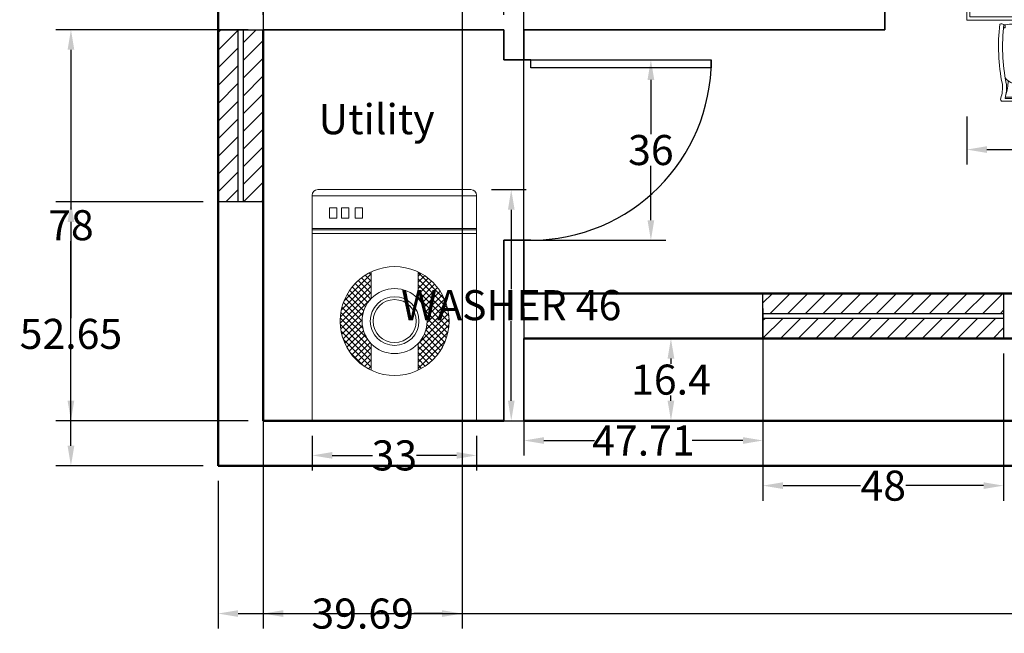
# Model space of a CAD drawing. Units: inches. Extents: x -1285 to -837, y -84 to 552.
# Tile 1 of 10: x -1285 to -1089, y -84 to 38. Entities that reach past the tile are written whole.
import ezdxf

# ---------------------------------------------------------------- set-up
doc = ezdxf.new("R2010")
doc.units = ezdxf.units.IN
doc.header["$MEASUREMENT"] = 0
for name, color, linetype, lineweight in [('A-ANNO-DIMS', 2, 'Continuous', 18), ('A-AREA-IDEN', 7, 'Continuous', 25), ('A-GLAZ-PATT', 191, 'Continuous', 13), ('Dining Table', 52, 'Continuous', 18), ('Doors', 34, 'Continuous', 25), ('Inner Wall', 202, 'Continuous', 35), ('Outer Wall', 12, 'Continuous', 50), ('Washing Machine', 133, 'Continuous', 18), ('Windows', 191, 'Continuous', 25)]:
    doc.layers.add(name, color=color, linetype=linetype, lineweight=lineweight)
doc.styles.get("Standard").update_dxf_attribs({"font": 'arial.ttf'})
doc.dimstyles.get("Standard").update_dxf_attribs({"dimtxt": 6, "dimasz": 4, "dimexe": 3, "dimexo": 3, "dimgap": 0.09, "dimtad": 0, "dimtih": 1, "dimtoh": 1, "dimdec": 1, "dimzin": 0, "dimdsep": 46, "dimlunit": 3, "dimtxsty": 'Standard', "dimcen": 0.09, "dimadec": 0, "dimazin": 0, "dimtfac": 1, "dimtdec": 1, "dimtofl": 0, "dimtmove": 0, "dimatfit": 3, "dimfxl": 1, "dimtolj": 1, "dimtzin": 0, "dimarcsym": 0})

# ---------------------------------------------------------------- blocks, each defined once
blk = doc.blocks.new('35')
for p, q in [((7268.4, 4404.4), (7268.4, 5204)), ((7288.4, 5224), (7831.6, 5224)), ((7851.6, 5204), (7851.6, 4404.4)), ((7268.4, 5201.6), (7851.6, 5201.6)), ((7329.8, 5159.5), (7355.7, 5159.5)), ((7329.8, 5122.5), (7329.8, 5159.5)), ((7355.7, 5159.5), (7355.7, 5122.5)), ((7372.4, 5159.5), (7398.4, 5159.5)), ((7372.4, 5122.5), (7372.4, 5159.5)), ((7398.4, 5159.5), (7398.4, 5122.5)), ((7420.7, 5159.5), (7446.7, 5159.5)), ((7420.7, 5122.5), (7420.7, 5159.5)), ((7446.7, 5159.5), (7446.7, 5122.5)), ((7355.7, 5122.5), (7329.8, 5122.5)), ((7398.4, 5122.5), (7372.4, 5122.5)), ((7446.7, 5122.5), (7420.7, 5122.5)), ((7268.4, 5085.6), (7851.6, 5085.6)), ((7268.4, 5080.8), (7851.6, 5080.8)), ((7268.4, 5068.6), (7851.6, 5068.6)), ((7381.6, 4829.3), (7477.8, 4925.5)), ((7477.8, 4921.2), (7470.7, 4928.4)), ((7477.8, 4837.6), (7477.8, 4932)), ((7644, 4837.6), (7644, 4932)), ((7737.2, 4836.4), (7644, 4929.6)), ((7644, 4917.1), (7653.8, 4926.9)), ((7372.1, 4798), (7477.8, 4903.7)), ((7418, 4887.6), (7431, 4900.5)), ((7476, 4835.7), (7421, 4890.8)), ((7477.8, 4855.8), (7432.1, 4901.5)), ((7477.8, 4877.6), (7444, 4911.4)), ((7477.8, 4899.4), (7456.9, 4920.3)), ((7644, 4895.3), (7667.4, 4918.7)), ((7644, 4873.5), (7680.1, 4909.6)), ((7748.5, 4803.3), (7644, 4907.8)), ((7644, 4851.7), (7691.9, 4899.5)), ((7368, 4750.2), (7477.8, 4860)), ((7368.4, 4772.5), (7477.8, 4881.9)), ((7458.1, 4810), (7401.5, 4866.6)), ((7466.3, 4823.6), (7410.8, 4879.1)), ((7753, 4777), (7644, 4886)), ((7753.9, 4754.2), (7644, 4864.2)), ((7647.7, 4833.6), (7702.8, 4888.6)), ((7657.2, 4821.2), (7712.8, 4876.8)), ((7665, 4807.2), (7722, 4864.2)), ((7369.8, 4730.2), (7477.8, 4838.2)), ((7445.6, 4757.1), (7379.3, 4823.3)), ((7447.2, 4777.2), (7385.7, 4838.8)), ((7451.7, 4794.6), (7393.1, 4853.2)), ((7752.5, 4733.8), (7644, 4842.3)), ((7671.1, 4791.5), (7730.2, 4850.6)), ((7675.1, 4773.7), (7737.4, 4836)), ((7676.1, 4752.8), (7743.5, 4820.3)), ((7464.3, 4694.7), (7370.3, 4788.7)), ((7373.3, 4711.9), (7449.7, 4788.3)), ((7448.4, 4732.4), (7374.1, 4806.7)), ((7644, 4677.1), (7752, 4785.1)), ((7749.3, 4715.3), (7670.3, 4794.2)), ((7672, 4727), (7748.5, 4803.4)), ((7477.8, 4659.4), (7368.2, 4769)), ((7378.3, 4695), (7445.7, 4762.5)), ((7644, 4655.3), (7753.8, 4765.1)), ((7744.6, 4698.1), (7675.9, 4766.8)), ((7477.8, 4637.6), (7368.1, 4747.3)), ((7477.8, 4615.7), (7371.1, 4722.5)), ((7384.4, 4679.4), (7446.7, 4741.7)), ((7391.6, 4664.8), (7450.7, 4723.8)), ((7644, 4633.4), (7753.4, 4742.9)), ((7644, 4611.6), (7749.7, 4717.3)), ((7731.6, 4667.4), (7672.1, 4727)), ((7738.6, 4682.2), (7675.6, 4745.3)), ((7477.8, 4593.9), (7379.1, 4692.6)), ((7399.9, 4651.2), (7456.8, 4708.1)), ((7409, 4638.5), (7464.7, 4694.1)), ((7419, 4626.7), (7474.1, 4681.8)), ((7644, 4589.8), (7740.2, 4686)), ((7704.7, 4628.9), (7649.6, 4684)), ((7714.6, 4640.8), (7658.7, 4696.7)), ((7723.6, 4653.7), (7666.3, 4710.9)), ((7450.9, 4599), (7402.3, 4647.6)), ((7430, 4615.8), (7477.8, 4663.6)), ((7477.8, 4583.4), (7477.8, 4677.7)), ((7644, 4583.4), (7644, 4677.7)), ((7694, 4617.8), (7644, 4667.8)), ((7682.3, 4607.6), (7644, 4645.9)), ((7441.7, 4605.8), (7477.8, 4641.8)), ((7454.4, 4596.6), (7477.8, 4620)), ((7669.8, 4598.3), (7644, 4624.1)), ((7691.5, 4615.5), (7703.1, 4627.1)), ((7468, 4588.4), (7477.8, 4598.2)), ((7656.4, 4589.9), (7644, 4602.3)), ((7851.6, 4404.4), (7268.4, 4404.4))]:
    blk.add_line(p, q)
for radius in [193.1, 115.3, 86.4, 76.4]:
    blk.add_circle((7560.9, 4757.7), radius)
for centre, start, end in [((7288.4, 5204), 90, 180), ((7831.6, 5204), 0, 90)]:
    blk.add_arc(centre, 20, start, end)
blk = doc.blocks.new('A$C51F1')
at = {"color": 0}
for p, q in [((0.2273, 0.4758), (0.0436, 0.4758)), ((0.2273, 0.4676), (0.0439, 0.4676)), ((0.2273, 0.4668), (0.0439, 0.4668)), ((0.2273, 0.4758), (0.4111, 0.4758)), ((0.2273, 0.4676), (0.4107, 0.4676)), ((0.2273, 0.4668), (0.4107, 0.4668)), ((0.2273, 0.3858), (0.1205, 0.3858)), ((0.2273, 0.3858), (0.3341, 0.3858)), ((0.0417, 0.0321), (0.0321, 0.0321)), ((0.0417, 0.0321), (0.0326, 0.0278)), ((0.0435, 0.0127), (0.0417, 0.0321)), ((0.4112, 0.0127), (0.4129, 0.0321)), ((0.4129, 0.0321), (0.4225, 0.0321)), ((0.4129, 0.0321), (0.4221, 0.0278))]:
    blk.add_line(p, q, dxfattribs=at)
blk.add_lwpolyline([(0.4387, 0.4737, 0.102523), (0.4291, 0.3863, -0.080461), (0.4447, 0.0091, -0.3023), (0.4203, 0.012, 0.197932), (0.4111, 0.0127, -0.028193), (0.3571, 0.0091), (0.227, 0.0091), (0.097, 0.0091, -0.028193), (0.0429, 0.0127, 0.197932), (0.0338, 0.012, -0.3023), (0.0093, 0.0091, -0.080461), (0.0249, 0.3863, 0.102523), (0.0153, 0.4737, -0.587111), (0.0261, 0.4929), (0.4279, 0.4929, -0.587111)], format="xyb", close=True, dxfattribs=at)
for centre, radius, start, end in [((0.044, 0.4735), 0.00242, 100.34496, 201.37417), ((-0.1898, 0.4063), 0.2409, 354.55133, 15.96258), ((0.0439, 0.4669), 0.000725, 87.37617, 197.52085), ((0.0438, 0.4664), 0.000433, 71.7715, 189.22024), ((-0.2563, 0.3584), 0.3173, 1.15909, 17.56409), ((0.7109, 0.3584), 0.3173, 162.43591, 178.84091), ((0.6445, 0.4063), 0.2409, 164.03742, 185.44867), ((0.4107, 0.4669), 0.000725, 342.47915, 92.62383), ((0.4109, 0.4664), 0.000433, 350.77976, 108.2285), ((0.4106, 0.4735), 0.00242, 338.62583, 79.65504), ((1.1806, 0.1494), 1.1544, 168.43567, 186.83625), ((0.1214, 0.2879), 0.0978, 90.51639, 143.19267), ((0.3332, 0.2879), 0.0978, 36.80733, 89.48361), ((-0.7259, 0.1494), 1.1544, 353.16375, 11.56433), ((0.0397, 0.0013), 0.012, 71.75361, 116.5375), ((0.4149, 0.0013), 0.012, 63.4625, 108.24639)]:
    blk.add_arc(centre, radius, start, end, dxfattribs=at)
blk = doc.blocks.new('Dining Table')
at = {"color": 0, "ltscale": 0.5}
for points in [[(5887.4, 1648.9), (7887.4, 1648.9), (7887.4, 2648.9), (5887.4, 2648.9)], [(5907.4, 1668.9), (7867.4, 1668.9), (7867.4, 2628.9), (5907.4, 2628.9)]]:
    blk.add_lwpolyline(points, close=True, dxfattribs=at)
at = {"color": 0, "ltscale": 0.5, "yscale": 1000, "zscale": 1000}
for p, xscale in [((6085.4, 2664.8), 1000), ((6685.4, 2664.8), 1000), ((7739.4, 2664.8), -1000)]:
    blk.add_blockref('A$C51F1', p, dxfattribs=dict(at, xscale=xscale))
at = {"color": 0, "ltscale": 0.5, "yscale": 1000, "zscale": 1000, "rotation": 180}
for p, xscale in [((6085.4, 1633), -1000), ((6685.4, 1633), -1000), ((7739.4, 1633), 1000)]:
    blk.add_blockref('A$C51F1', p, dxfattribs=dict(at, xscale=xscale))
blk = doc.blocks.new('*U17')
for p, q in [((-40, 0), (-40, 6)), ((0, 0), (0, 6))]:
    blk.add_line(p, q)
blk.add_lwpolyline([(0, 0), (0, -40), (-1.75, -40), (-1.75, 0)], close=True)
blk.add_arc((0, 0), 40, 180, 270)
blk = doc.blocks.new('WIN-34x9')
for p, q in [((4, 0), (4, 34.35)), ((5, 34.35), (5, 0))]:
    blk.add_line(p, q)
blk.add_lwpolyline([(9, 34.35), (9, 0), (0, 0), (0, 34.35)], close=True)
blk = doc.blocks.new('*D53')
at = {"layer": 'A-ANNO-DIMS', "color": 0, "lineweight": -2, "transparency": 16777216}
for p, q in [((-1190.95, 4.04), (-1184.04, 4.04)), ((-1187.04, 0.04), (-1187.04, -15.82)), ((-1187.04, -38.06), (-1187.04, -22.2)), ((-1190.95, -42.06), (-1184.04, -42.06))]:
    blk.add_line(p, q, dxfattribs=at)
at = {"layer": 'A-ANNO-DIMS', "color": 0, "transparency": 16777216}
for points in [[(-1187.7, 0.04), (-1186.37, 0.04), (-1187.04, 4.04)], [(-1187.7, -38.06), (-1186.37, -38.06), (-1187.04, -42.06)]]:
    blk.add_solid(points, dxfattribs=at)
at = {"layer": 'Defpoints', "color": 0, "transparency": 16777216}
for p in [(-1193.95, 4.04), (-1187.04, 4.04), (-1193.95, -42.06)]:
    blk.add_point(p, dxfattribs=at)
at = {"layer": 'A-ANNO-DIMS', "color": 0, "transparency": 16777216, "insert": (-1187.04, -19.01), "char_height": 6, "attachment_point": 5}
blk.add_mtext('\\A1;WASHER 46', dxfattribs=at)
blk = doc.blocks.new('*D54')
at = {"layer": 'A-ANNO-DIMS', "color": 0, "lineweight": -2, "transparency": 16777216}
for p, q in [((-1226.76, -45.06), (-1226.76, -51.98)), ((-1193.95, -45.06), (-1193.95, -51.98)), ((-1222.76, -48.98), (-1214.74, -48.98)), ((-1197.95, -48.98), (-1205.97, -48.98))]:
    blk.add_line(p, q, dxfattribs=at)
at = {"layer": 'A-ANNO-DIMS', "color": 0, "transparency": 16777216}
for points in [[(-1222.76, -48.31), (-1222.76, -49.64), (-1226.76, -48.98)], [(-1197.95, -48.31), (-1197.95, -49.64), (-1193.95, -48.98)]]:
    blk.add_solid(points, dxfattribs=at)
at = {"layer": 'Defpoints', "color": 0, "transparency": 16777216}
for p in [(-1226.76, -42.06), (-1193.95, -42.06), (-1193.95, -48.98)]:
    blk.add_point(p, dxfattribs=at)
at = {"layer": 'A-ANNO-DIMS', "color": 0, "transparency": 16777216, "insert": (-1210.36, -48.98), "char_height": 6, "attachment_point": 5}
blk.add_mtext('\\A1;33', dxfattribs=at)
blk = doc.blocks.new('*D58')
at = {"layer": 'A-ANNO-DIMS', "color": 0, "lineweight": -2, "transparency": 16777216}
for p, q in [((-1096.15, 18.66), (-1096.15, 9.03)), ((-1032.53, 18.66), (-1032.53, 9.03)), ((-1092.15, 12.03), (-1068.73, 12.03)), ((-1036.53, 12.03), (-1059.95, 12.03))]:
    blk.add_line(p, q, dxfattribs=at)
at = {"layer": 'A-ANNO-DIMS', "color": 0, "transparency": 16777216}
for points in [[(-1092.15, 12.7), (-1092.15, 11.36), (-1096.15, 12.03)], [(-1036.53, 12.7), (-1036.53, 11.36), (-1032.53, 12.03)]]:
    blk.add_solid(points, dxfattribs=at)
at = {"layer": 'Defpoints', "color": 0, "transparency": 16777216}
for p in [(-1096.15, 21.66), (-1032.53, 21.66), (-1032.53, 12.03)]:
    blk.add_point(p, dxfattribs=at)
at = {"layer": 'A-ANNO-DIMS', "color": 0, "transparency": 16777216, "insert": (-1064.34, 12.03), "char_height": 6, "attachment_point": 5}
blk.add_mtext('\\A1;64', dxfattribs=at)
blk = doc.blocks.new('*D69')
at = {"layer": 'A-ANNO-DIMS', "color": 0, "lineweight": -2, "transparency": 16777216}
for p, q in [((-1245.53, -54.06), (-1245.53, -83.53)), ((-877.53, -54.06), (-877.53, -83.53)), ((-1241.53, -80.53), (-1068.25, -80.53)), ((-881.53, -80.53), (-1054.81, -80.53))]:
    blk.add_line(p, q, dxfattribs=at)
at = {"layer": 'A-ANNO-DIMS', "color": 0, "transparency": 16777216}
for points in [[(-1241.53, -79.86), (-1241.53, -81.2), (-1245.53, -80.53)], [(-881.53, -79.86), (-881.53, -81.2), (-877.53, -80.53)]]:
    blk.add_solid(points, dxfattribs=at)
at = {"layer": 'Defpoints', "color": 0, "transparency": 16777216}
for p in [(-1245.53, -51.06), (-877.53, -51.06), (-877.53, -80.53)]:
    blk.add_point(p, dxfattribs=at)
at = {"layer": 'A-ANNO-DIMS', "color": 0, "transparency": 16777216, "insert": (-1061.53, -80.53), "char_height": 6, "attachment_point": 5}
blk.add_mtext('\\A1;368', dxfattribs=at)
blk = doc.blocks.new('*D77')
at = {"layer": 'A-ANNO-DIMS', "color": 0, "lineweight": -2, "transparency": 16777216}
for p, q in [((-1239.53, 35.94), (-1277.88, 35.94)), ((-1274.88, 31.94), (-1274.88, 0.09)), ((-1274.88, -38.06), (-1274.88, -6.21)), ((-1239.53, -42.06), (-1277.88, -42.06))]:
    blk.add_line(p, q, dxfattribs=at)
at = {"layer": 'A-ANNO-DIMS', "color": 0, "transparency": 16777216}
for points in [[(-1275.55, 31.94), (-1274.21, 31.94), (-1274.88, 35.94)], [(-1275.55, -38.06), (-1274.21, -38.06), (-1274.88, -42.06)]]:
    blk.add_solid(points, dxfattribs=at)
at = {"layer": 'Defpoints', "color": 0, "transparency": 16777216}
for p in [(-1274.88, 35.94), (-1236.53, 35.94), (-1236.53, -42.06)]:
    blk.add_point(p, dxfattribs=at)
at = {"layer": 'A-ANNO-DIMS', "color": 0, "transparency": 16777216, "insert": (-1274.88, -3.06), "char_height": 6, "attachment_point": 5}
blk.add_mtext('\\A1;78', dxfattribs=at)
blk = doc.blocks.new('*D79')
at = {"layer": 'A-ANNO-DIMS', "color": 0, "lineweight": -2, "transparency": 16777216}
for p, q in [((-1236.53, 38.94), (-1236.53, 551.29)), ((-1188.53, 38.94), (-1188.53, 551.29)), ((-1232.53, 548.29), (-1217.04, 548.29)), ((-1192.53, 548.29), (-1208.02, 548.29))]:
    blk.add_line(p, q, dxfattribs=at)
at = {"layer": 'A-ANNO-DIMS', "color": 0, "transparency": 16777216}
for points in [[(-1232.53, 548.96), (-1232.53, 547.62), (-1236.53, 548.29)], [(-1192.53, 548.96), (-1192.53, 547.62), (-1188.53, 548.29)]]:
    blk.add_solid(points, dxfattribs=at)
at = {"layer": 'Defpoints', "color": 0, "transparency": 16777216}
for p in [(-1188.53, 548.29), (-1236.53, 35.94), (-1188.53, 35.94)]:
    blk.add_point(p, dxfattribs=at)
at = {"layer": 'A-ANNO-DIMS', "color": 0, "transparency": 16777216, "insert": (-1212.53, 548.29), "char_height": 6, "attachment_point": 5}
blk.add_mtext('\\A1;48', dxfattribs=at)
blk = doc.blocks.new('*D80')
at = {"layer": 'A-ANNO-DIMS', "color": 0, "lineweight": -2, "transparency": 16777216}
for p, q in [((-1184.53, -13.66), (-1184.53, 551.29)), ((-1032.53, -13.66), (-1032.53, 551.29)), ((-1180.53, 548.29), (-1114.94, 548.29)), ((-1036.53, 548.29), (-1102.12, 548.29))]:
    blk.add_line(p, q, dxfattribs=at)
at = {"layer": 'A-ANNO-DIMS', "color": 0, "transparency": 16777216}
for points in [[(-1180.53, 548.96), (-1180.53, 547.62), (-1184.53, 548.29)], [(-1036.53, 548.96), (-1036.53, 547.62), (-1032.53, 548.29)]]:
    blk.add_solid(points, dxfattribs=at)
at = {"layer": 'Defpoints', "color": 0, "transparency": 16777216}
for p in [(-1032.53, 548.29), (-1184.53, -16.66), (-1032.53, -16.66)]:
    blk.add_point(p, dxfattribs=at)
at = {"layer": 'A-ANNO-DIMS', "color": 0, "transparency": 16777216, "insert": (-1108.53, 548.29), "char_height": 6, "attachment_point": 5}
blk.add_mtext('\\A1;152', dxfattribs=at)
blk = doc.blocks.new('*D96')
at = {"layer": 'A-ANNO-DIMS', "color": 0, "lineweight": -2, "transparency": 16777216}
for p, q in [((-1236.53, 506.94), (-1236.53, -83.53)), ((-1196.84, 506.94), (-1196.84, -83.53)), ((-1232.53, -80.53), (-1226.9, -80.53)), ((-1200.84, -80.53), (-1206.47, -80.53))]:
    blk.add_line(p, q, dxfattribs=at)
at = {"layer": 'A-ANNO-DIMS', "color": 0, "transparency": 16777216}
for points in [[(-1232.53, -79.86), (-1232.53, -81.2), (-1236.53, -80.53)], [(-1200.84, -79.86), (-1200.84, -81.2), (-1196.84, -80.53)]]:
    blk.add_solid(points, dxfattribs=at)
at = {"layer": 'Defpoints', "color": 0, "transparency": 16777216}
for p in [(-1236.53, 509.94), (-1196.84, 509.94), (-1196.84, -80.53)]:
    blk.add_point(p, dxfattribs=at)
at = {"layer": 'A-ANNO-DIMS', "color": 0, "transparency": 16777216, "insert": (-1216.68, -80.53), "char_height": 6, "attachment_point": 5}
blk.add_mtext('\\A1;39.69', dxfattribs=at)
blk = doc.blocks.new('*D100')
at = {"layer": 'A-ANNO-DIMS', "color": 0, "lineweight": -2, "transparency": 16777216}
for p, q in [((-1184.53, -19.66), (-1184.53, -49.01)), ((-1136.82, -19.66), (-1136.82, -49.01)), ((-1180.53, -46.01), (-1170.43, -46.01)), ((-1140.82, -46.01), (-1150.92, -46.01))]:
    blk.add_line(p, q, dxfattribs=at)
at = {"layer": 'A-ANNO-DIMS', "color": 0, "transparency": 16777216}
for points in [[(-1180.53, -45.34), (-1180.53, -46.68), (-1184.53, -46.01)], [(-1140.82, -45.34), (-1140.82, -46.68), (-1136.82, -46.01)]]:
    blk.add_solid(points, dxfattribs=at)
at = {"layer": 'Defpoints', "color": 0, "transparency": 16777216}
for p in [(-1184.53, -16.66), (-1136.82, -16.66), (-1184.53, -46.01)]:
    blk.add_point(p, dxfattribs=at)
at = {"layer": 'A-ANNO-DIMS', "color": 0, "transparency": 16777216, "insert": (-1160.67, -46.01), "char_height": 6, "attachment_point": 5}
blk.add_mtext('\\A1;47.71', dxfattribs=at)
blk = doc.blocks.new('*D101')
at = {"layer": 'A-ANNO-DIMS', "color": 0, "lineweight": -2, "transparency": 16777216}
for p, q in [((-1136.82, -28.66), (-1136.82, -58.01)), ((-1088.82, -28.66), (-1088.82, -58.01)), ((-1132.82, -55.01), (-1117.33, -55.01)), ((-1092.82, -55.01), (-1108.3, -55.01))]:
    blk.add_line(p, q, dxfattribs=at)
at = {"layer": 'A-ANNO-DIMS', "color": 0, "transparency": 16777216}
for points in [[(-1132.82, -54.34), (-1132.82, -55.68), (-1136.82, -55.01)], [(-1092.82, -54.34), (-1092.82, -55.68), (-1088.82, -55.01)]]:
    blk.add_solid(points, dxfattribs=at)
at = {"layer": 'Defpoints', "color": 0, "transparency": 16777216}
for p in [(-1136.82, -25.66), (-1088.82, -25.66), (-1136.82, -55.01)]:
    blk.add_point(p, dxfattribs=at)
at = {"layer": 'A-ANNO-DIMS', "color": 0, "transparency": 16777216, "insert": (-1112.82, -55.01), "char_height": 6, "attachment_point": 5}
blk.add_mtext('\\A1;48', dxfattribs=at)
blk = doc.blocks.new('*D110')
at = {"layer": 'A-ANNO-DIMS', "color": 0, "lineweight": -2, "transparency": 16777216}
for p, q in [((-1185.53, 29.94), (-1156.18, 29.94)), ((-1159.18, 25.94), (-1159.18, 15.09)), ((-1159.18, -2.06), (-1159.18, 8.78)), ((-1185.53, -6.06), (-1156.18, -6.06))]:
    blk.add_line(p, q, dxfattribs=at)
at = {"layer": 'A-ANNO-DIMS', "color": 0, "transparency": 16777216}
for points in [[(-1159.85, 25.94), (-1158.51, 25.94), (-1159.18, 29.94)], [(-1159.85, -2.06), (-1158.51, -2.06), (-1159.18, -6.06)]]:
    blk.add_solid(points, dxfattribs=at)
at = {"layer": 'Defpoints', "color": 0, "transparency": 16777216}
for p in [(-1188.53, 29.94), (-1188.53, -6.06), (-1159.18, -6.06)]:
    blk.add_point(p, dxfattribs=at)
at = {"layer": 'A-ANNO-DIMS', "color": 0, "transparency": 16777216, "insert": (-1159.18, 11.94), "char_height": 6, "attachment_point": 5}
blk.add_mtext('\\A1;36', dxfattribs=at)
blk = doc.blocks.new('*D115')
at = {"layer": 'A-ANNO-DIMS', "color": 0, "lineweight": -2, "transparency": 16777216}
for p, q in [((-1248.53, 1.59), (-1277.88, 1.59)), ((-1274.88, -2.41), (-1274.88, -21.58)), ((-1274.88, -47.06), (-1274.88, -27.89)), ((-1248.53, -51.06), (-1277.88, -51.06))]:
    blk.add_line(p, q, dxfattribs=at)
at = {"layer": 'A-ANNO-DIMS', "color": 0, "transparency": 16777216}
for points in [[(-1275.55, -2.41), (-1274.21, -2.41), (-1274.88, 1.59)], [(-1275.55, -47.06), (-1274.21, -47.06), (-1274.88, -51.06)]]:
    blk.add_solid(points, dxfattribs=at)
at = {"layer": 'Defpoints', "color": 0, "transparency": 16777216}
for p in [(-1274.88, 1.59), (-1245.53, 1.59), (-1245.53, -51.06)]:
    blk.add_point(p, dxfattribs=at)
at = {"layer": 'A-ANNO-DIMS', "color": 0, "transparency": 16777216, "insert": (-1274.88, -24.74), "char_height": 6, "attachment_point": 5}
blk.add_mtext('\\A1;52.65', dxfattribs=at)
blk = doc.blocks.new('*D120')
at = {"layer": 'A-ANNO-DIMS', "color": 0, "lineweight": -2, "transparency": 16777216}
for p, q in [((-1181.53, -25.66), (-1152.18, -25.66)), ((-1155.18, -29.66), (-1155.18, -30.71)), ((-1155.18, -38.06), (-1155.18, -37.01)), ((-1181.53, -42.06), (-1152.18, -42.06))]:
    blk.add_line(p, q, dxfattribs=at)
at = {"layer": 'A-ANNO-DIMS', "color": 0, "transparency": 16777216}
for points in [[(-1155.85, -29.66), (-1154.51, -29.66), (-1155.18, -25.66)], [(-1155.85, -38.06), (-1154.51, -38.06), (-1155.18, -42.06)]]:
    blk.add_solid(points, dxfattribs=at)
at = {"layer": 'Defpoints', "color": 0, "transparency": 16777216}
for p in [(-1184.53, -25.66), (-1184.53, -42.06), (-1155.18, -42.06)]:
    blk.add_point(p, dxfattribs=at)
at = {"layer": 'A-ANNO-DIMS', "color": 0, "transparency": 16777216, "insert": (-1155.18, -33.86), "char_height": 6, "attachment_point": 5}
blk.add_mtext('\\A1;16.4', dxfattribs=at)

msp = doc.modelspace()

# ---------------------------------------------------------------- hatches: boundary and pattern name
at = {"layer": 'A-GLAZ-PATT'}
h = msp.add_hatch(dxfattribs=at)
h.set_pattern_fill('ANSI31', color=256, scale=20)
h.set_pattern_definition([(45, (-2191.666, -702.1458), (-1.767767, 1.767767), [])])
h.paths.add_polyline_path([(-921.1945, 518.9392), (-984.2307, 518.9392), (-984.2307, 514.9392), (-921.1945, 514.9392)])
h.paths.add_polyline_path([(-921.1945, 513.9392), (-984.2307, 513.9392), (-984.2307, 509.9392), (-921.1945, 509.9392)])
h.paths.add_polyline_path([(-877.5299, 480.0491), (-881.5299, 480.0491), (-881.5299, 417.0129), (-877.5299, 417.0129)])
h.paths.add_polyline_path([(-882.5299, 480.0491), (-886.5299, 480.0491), (-886.5299, 417.0129), (-882.5299, 417.0129)])
h.paths.add_polyline_path([(-877.5299, 356.1195), (-881.5299, 356.1195), (-881.5299, 321.7709), (-877.5299, 321.7709)])
h.paths.add_polyline_path([(-882.5299, 356.1195), (-886.5299, 356.1195), (-886.5299, 321.7709), (-882.5299, 321.7709)])
h.paths.add_polyline_path([(-1133.8033, 518.9392), (-1196.8396, 518.9392), (-1196.8396, 514.9392), (-1133.8033, 514.9392)])
h.paths.add_polyline_path([(-1133.8033, 513.9392), (-1196.8396, 513.9392), (-1196.8396, 509.9392), (-1133.8033, 509.9392)])
h.paths.add_polyline_path([(-1236.5299, 138.1751), (-1240.5299, 138.1751), (-1240.5299, 75.1388), (-1236.5299, 75.1388)])
h.paths.add_polyline_path([(-1241.5299, 138.1751), (-1245.5299, 138.1751), (-1245.5299, 75.1388), (-1241.5299, 75.1388)])
h.paths.add_polyline_path([(-1236.5299, 35.9392), (-1240.5299, 35.9392), (-1240.5299, 1.5906), (-1236.5299, 1.5906)])
h.paths.add_polyline_path([(-1241.5299, 35.9392), (-1245.5299, 35.9392), (-1245.5299, 1.5906), (-1241.5299, 1.5906)])
h.paths.add_polyline_path([(-1088.8155, -16.6608), (-1136.8155, -16.6608), (-1136.8155, -20.6608), (-1088.8155, -20.6608)])
h.paths.add_polyline_path([(-1088.8155, -21.6608), (-1136.8155, -21.6608), (-1136.8155, -25.6608), (-1088.8155, -25.6608)])

# ---------------------------------------------------------------- linework, layer by layer
at = {"layer": 'Inner Wall'}
for p, q in [((-1112.5299, 104.7212), (-1112.5299, 35.9392)), ((-1236.5299, 35.9392), (-1188.5299, 35.9392)), ((-1188.5299, 35.9392), (-1188.5299, 29.9392)), ((-1184.5299, 35.9392), (-1184.5299, 29.9392)), ((-1184.5299, 35.9392), (-1112.5299, 35.9392)), ((-1188.5299, 29.9392), (-1184.5299, 29.9392)), ((-1188.5299, -6.0608), (-1184.5299, -6.0608)), ((-1188.5299, -6.0608), (-1188.5299, -42.0608)), ((-1184.5299, -6.0608), (-1184.5299, -16.6608)), ((-1184.5299, -25.6608), (-1184.5299, -42.0608))]:
    msp.add_line(p, q, dxfattribs=at)
at = {"layer": 'Outer Wall'}
for p, q in [((-1245.5299, 518.9392), (-1245.5299, -51.0608)), ((-1236.5299, 35.9392), (-1236.5299, -42.0608)), ((-1184.5299, -16.6608), (-1032.5299, -16.6608)), ((-1184.5299, -25.6608), (-1032.5299, -25.6608)), ((-1236.5299, -42.0608), (-1188.5299, -42.0608)), ((-1184.5299, -42.0608), (-1032.5299, -42.0608)), ((-1245.5299, -51.0608), (-968.24, -51.0608))]:
    msp.add_line(p, q, dxfattribs=at)
at = {"layer": 'Windows'}
for p, q in [((-1136.8155, -20.6608), (-1088.8155, -20.6608)), ((-1088.8155, -21.6608), (-1136.8155, -21.6608))]:
    msp.add_line(p, q, dxfattribs=at)
msp.add_lwpolyline([(-1088.8155, -16.6608), (-1088.8155, -25.6608), (-1136.8155, -25.6608), (-1136.8155, -16.6608)], close=True, dxfattribs=at)

# ---------------------------------------------------------------- block references
at = {"layer": 'Dining Table', "xscale": 0.0318116679632498, "yscale": 0.0318116679632498, "zscale": 0.0318116679632498}
msp.add_blockref('Dining Table', (-1283.4424, -14.6094), dxfattribs=at)
at = {"layer": 'Doors', "xscale": 0.9, "yscale": 0.9, "zscale": 0.9, "rotation": 90}
msp.add_blockref('*U17', (-1183.1299, 29.9392), dxfattribs=at)
at = {"layer": 'Washing Machine', "xscale": 0.0562533047698356, "yscale": 0.0562533047698356, "zscale": 0.0562533047698356}
msp.add_blockref('35', (-1635.6318, -289.8256), dxfattribs=at)
at = {"layer": 'Windows'}
msp.add_blockref('WIN-34x9', (-1245.53, 1.5907), dxfattribs=at)

# ---------------------------------------------------------------- texts
at = {"layer": 'A-AREA-IDEN', "insert": (-1248.2983, 21.0895), "char_height": 6, "attachment_point": 1}
msp.add_mtext_dynamic_manual_height_columns('\\pxqc;Utility', width=68.784729, gutter_width=1, heights=[0], dxfattribs=at)

# ---------------------------------------------------------------- dimensions: what is measured, and where the dimension line sits
at = {"layer": 'A-ANNO-DIMS'}
for base, p1, p2, override, picture, middle in [((-1188.5299, 548.2892), (-1236.5299, 35.9392), (-1188.5299, 35.9392), {"dimdec": 0, "dimlfac": 1, "dimrnd": 0, "dimzin": 0, "dimdsep": 46, "dimlunit": 2}, '*D79', (-1212.5299, 548.2892)), ((-1032.5299, 548.2892), (-1184.5299, -16.6608), (-1032.5299, -16.6608), {"dimdec": 0, "dimlfac": 1, "dimrnd": 0, "dimzin": 0, "dimdsep": 46, "dimlunit": 2}, '*D80', (-1108.5299, 548.2892)), ((-1196.8396, -80.5308), (-1236.5299, 509.9392), (-1196.8396, 509.9392), {"dimdec": 2, "dimlfac": 1, "dimrnd": 0, "dimzin": 0, "dimdsep": 46, "dimlunit": 2}, '*D96', (-1216.6847, -80.5308)), ((-1032.5299, 12.0299), (-1096.1532, 21.6576), (-1032.5299, 21.6576), {"dimdec": 0, "dimlfac": 1, "dimrnd": 0, "dimzin": 0, "dimdsep": 46, "dimlunit": 2}, '*D58', (-1064.3415, 12.0299)), ((-1193.9532, -48.9765), (-1226.7601, -42.0608), (-1193.9532, -42.0608), {"dimdec": 0, "dimlfac": 1, "dimrnd": 0, "dimzin": 0, "dimdsep": 46, "dimlunit": 2}, '*D54', (-1210.3567, -48.9765)), ((-877.5299, -80.5308), (-1245.5299, -51.0608), (-877.5299, -51.0608), {"dimdec": 0, "dimlfac": 1, "dimrnd": 0, "dimzin": 0, "dimdsep": 46, "dimlunit": 2}, '*D69', (-1061.5299, -80.5308))]:
    dim = msp.add_linear_dim(base=base, p1=p1, p2=p2, dimstyle='Standard', override=override, dxfattribs=at)
    dim.commit()
    dim.dimension.update_dxf_attribs({"geometry": picture, "text_midpoint": middle})
for base, p1, p2, angle, override, picture, middle in [((-1274.8799, 35.9392), (-1236.5299, -42.0608), (-1236.5299, 35.9392), 90, {"dimdec": 0, "dimlfac": 1, "dimrnd": 0, "dimzin": 0, "dimdsep": 46, "dimlunit": 2}, '*D77', (-1274.8799, -3.0608)), ((-1159.1799, -6.0608), (-1188.5299, 29.9392), (-1188.5299, -6.0608), 270, {"dimdec": 0, "dimlfac": 1, "dimrnd": 0, "dimzin": 0, "dimdsep": 46, "dimlunit": 2}, '*D110', (-1159.1799, 11.9392)), ((-1274.8799, 1.5906), (-1245.5299, -51.0608), (-1245.5299, 1.5906), 90, {"dimdec": 2, "dimlfac": 1, "dimrnd": 0, "dimzin": 0, "dimdsep": 46, "dimlunit": 2}, '*D115', (-1274.8799, -24.7351)), ((-1184.5299, -46.0108), (-1136.8155, -16.6608), (-1184.5299, -16.6608), 180, {"dimdec": 2, "dimlfac": 1, "dimrnd": 0, "dimzin": 0, "dimdsep": 46, "dimlunit": 2}, '*D100', (-1160.6727, -46.0108)), ((-1155.1799, -42.0608), (-1184.5299, -25.6608), (-1184.5299, -42.0608), 270, {"dimdec": 1, "dimlfac": 1, "dimrnd": 0, "dimzin": 0, "dimdsep": 46, "dimlunit": 2}, '*D120', (-1155.1799, -33.8608)), ((-1136.8155, -55.0108), (-1088.8155, -25.6608), (-1136.8155, -25.6608), 180, {"dimdec": 0, "dimlfac": 1, "dimrnd": 0, "dimzin": 0, "dimdsep": 46, "dimlunit": 2}, '*D101', (-1112.8155, -55.0108))]:
    dim = msp.add_linear_dim(base=base, p1=p1, p2=p2, angle=angle, dimstyle='Standard', override=override, dxfattribs=at)
    dim.commit()
    dim.dimension.update_dxf_attribs({"geometry": picture, "text_midpoint": middle})
dim = msp.add_linear_dim(base=(-1187.0374, 4.0444), p1=(-1193.9532, -42.0608), p2=(-1193.9532, 4.0444), angle=90, text='WASHER <>', dimstyle='Standard', override={"dimdec": 0, "dimlfac": 1, "dimrnd": 0, "dimzin": 0, "dimdsep": 46, "dimlunit": 2}, dxfattribs=at)
dim.commit()
dim.dimension.update_dxf_attribs({"geometry": '*D53', "text_midpoint": (-1187.0374, -19.0082)})

doc.saveas('drawing.dxf')
